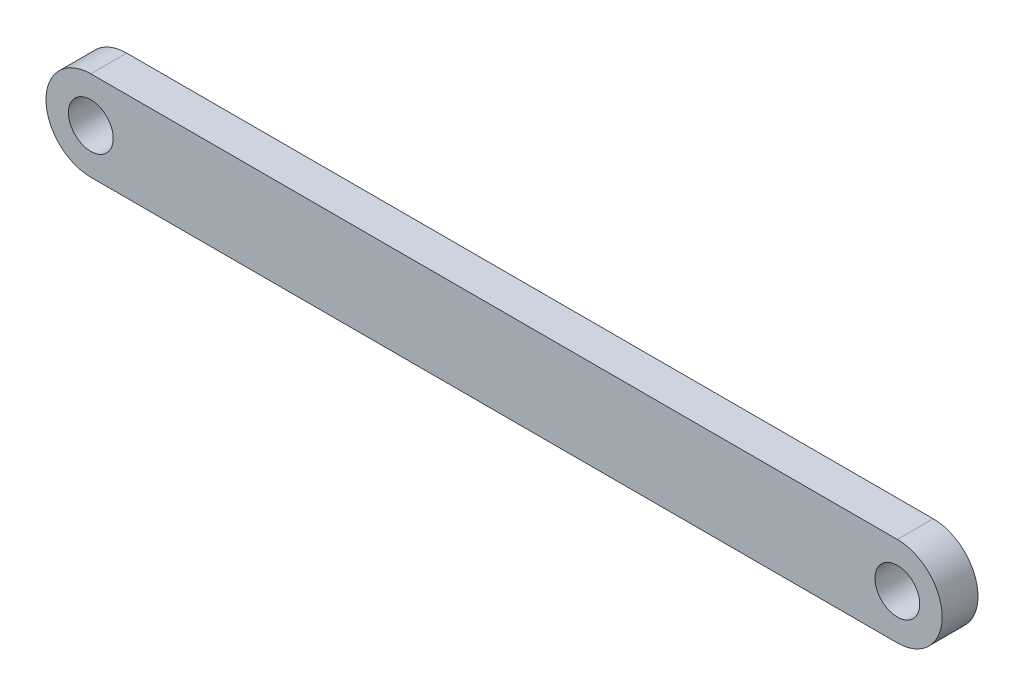
SolidWorks part; units mm, degrees
material "Plain Carbon Steel"
ref_plane "Front Plane" through (0, 0, 0) normal (0, 0, 1) x (1, 0, 0)
ref_plane "Top Plane" through (0, 0, 0) normal (0, 1, 0) x (1, 0, 0)
ref_plane "Right Plane" through (0, 0, 0) normal (1, 0, 0) x (0, 0, -1)
sketch "Link Profile Sketch" plane through (0, 0, 0) normal (0, 0, 1) x (1, 0, 0)
  line L0 (-45, 0) -> (45, 0) construction
  line L1 (-45, 5) -> (45, 5)
  line L2 (-45, -5) -> (45, -5)
  arc A0 (-45, 5) -> (-45, -5) centre (-45, 0) ccw
  arc A1 (45, -5) -> (45, 5) centre (45, 0) ccw
  circle A2 centre (-45, 0) radius 2.5
  circle A3 centre (45, 0) radius 2.5
  point P2 (0, 0)
  dimension "D2" = 5
  dimension "D3" = 5
  dimension "D4" = 5
  dimension "D1" = 90
extrude "Link Bar 4mm" add sketch "Link Profile Sketch" along normal mid plane 4
